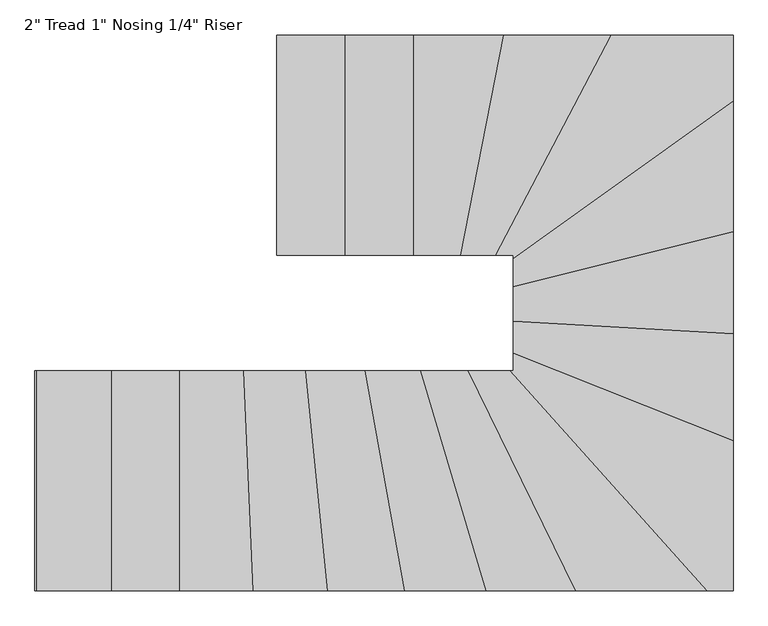
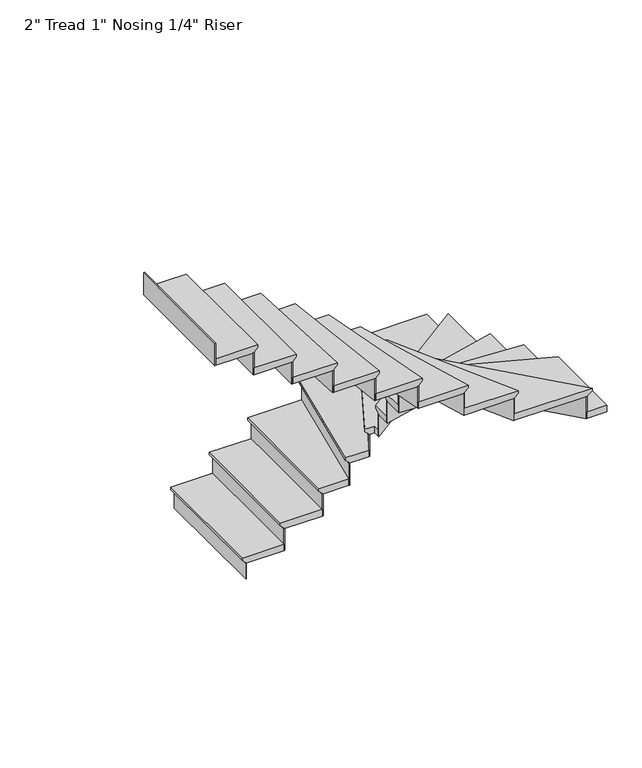
"""IFC4 building model written with IfcOpenShell, lengths in millimetres: stair flight geometry."""

from ifc_helpers import new_model, si_unit, origin, place, context, project, spatial, faceted_brep, source, transform, mapped, element, save


def stair_flight_52755f88(model_context):
    return source(origin(), model_context, "Body", "Brep", [
        faceted_brep([(158.6923968, 2024.0935985, 6551.0833333), (158.6923968, 2024.0935985, 6570.1333333), (158.6923968, 2922.8476133, 6570.1333333), (158.6923968, 2922.8476133, 6551.0833333), (184.0923968, 2024.0935985, 6525.6833333), (184.0923968, 2922.8476133, 6525.6833333), (463.4923968, 2024.0935985, 6570.1333333), (463.4923968, 2922.8476133, 6570.1333333), (184.0923968, 2922.8476133, 6519.3333333), (463.4923968, 2922.8476133, 6519.3333333), (463.4923968, 2024.0935985, 6519.3333333), (184.0923968, 2024.0935985, 6519.3333333)], [[[0, 1, 2, 3]], [[4, 0, 3, 5]], [[2, 1, 6, 7]], [[8, 9, 10, 11]], [[2, 7, 9, 8, 5, 3]], [[8, 11, 4, 5]], [[6, 1, 0, 4, 11, 10]], [[7, 6, 10, 9]]]),
        faceted_brep([(184.0923968, 2024.0935985, 6519.3333333), (184.0923968, 2024.0935985, 6400.8), (190.4423968, 2024.0935985, 6400.8), (190.4423968, 2024.0935985, 6519.3333333), (184.0923968, 2922.8476133, 6519.3333333), (190.4423968, 2922.8476133, 6519.3333333), (190.4423968, 2922.8476133, 6400.8), (184.0923968, 2922.8476133, 6400.8)], [[[0, 1, 2, 3]], [[4, 5, 6, 7]], [[1, 0, 4, 7]], [[2, 1, 7, 6]], [[3, 2, 6, 5]], [[0, 3, 5, 4]]]),
        faceted_brep([(463.4923968, 2024.0935985, 6688.6666667), (463.4923968, 2024.0935985, 6519.3333333), (469.8423968, 2024.0935985, 6519.3333333), (469.8423968, 2024.0935985, 6688.6666667), (463.4923968, 2922.8476133, 6688.6666667), (469.8423968, 2922.8476133, 6688.6666667), (469.8423968, 2922.8476133, 6519.3333333), (463.4923968, 2922.8476133, 6519.3333333)], [[[0, 1, 2, 3]], [[4, 5, 6, 7]], [[1, 0, 4, 7]], [[2, 1, 7, 6]], [[3, 2, 6, 5]], [[0, 3, 5, 4]]]),
        faceted_brep([(438.0923968, 2922.8476133, 6739.4666667), (438.0923968, 2024.0935985, 6739.4666667), (742.8923968, 2024.0935985, 6739.4666667), (742.8923968, 2922.8476133, 6739.4666667), (463.4923968, 2922.8476133, 6688.6666667), (742.8923968, 2922.8476133, 6688.6666667), (742.8923968, 2024.0935985, 6688.6666667), (463.4923968, 2024.0935985, 6688.6666667), (463.4923968, 2922.8476133, 6695.0166667), (438.0923968, 2922.8476133, 6720.4166667), (463.4923968, 2024.0935985, 6695.0166667), (438.0923968, 2024.0935985, 6720.4166667)], [[[0, 1, 2, 3]], [[4, 5, 6, 7]], [[0, 3, 5, 4, 8, 9]], [[4, 7, 10, 8]], [[2, 1, 11, 10, 7, 6]], [[3, 2, 6, 5]], [[11, 1, 0, 9]], [[10, 11, 9, 8]]]),
        faceted_brep([(742.8923968, 2024.0935985, 6858.0), (742.8923968, 2024.0935985, 6688.6666667), (749.2423968, 2024.0935985, 6688.6666667), (749.2423968, 2024.0935985, 6858.0), (742.8923968, 2922.8476133, 6858.0), (749.2423968, 2922.8476133, 6858.0), (749.2423968, 2922.8476133, 6688.6666667), (742.8923968, 2922.8476133, 6688.6666667)], [[[0, 1, 2, 3]], [[4, 5, 6, 7]], [[1, 0, 4, 7]], [[2, 1, 7, 6]], [[3, 2, 6, 5]], [[0, 3, 5, 4]]]),
        faceted_brep([(717.4923968, 2922.8476133, 6908.8), (717.4923968, 2024.0935985, 6908.8), (934.4682952, 2024.0935985, 6908.8), (1111.0881205, 2922.8476133, 6908.8), (742.8923968, 2922.8476133, 6858.0), (1111.0881205, 2922.8476133, 6858.0), (934.4682952, 2024.0935985, 6858.0), (742.8923968, 2024.0935985, 6858.0), (742.8923968, 2922.8476133, 6864.35), (717.4923968, 2922.8476133, 6889.75), (742.8923968, 2024.0935985, 6864.35), (717.4923968, 2024.0935985, 6889.75)], [[[0, 1, 2, 3]], [[4, 5, 6, 7]], [[0, 3, 5, 4, 8, 9]], [[4, 7, 10, 8]], [[2, 1, 11, 10, 7, 6]], [[3, 2, 6, 5]], [[11, 1, 0, 9]], [[10, 11, 9, 8]]]),
        faceted_brep([(934.4682952, 2024.0935985, 7027.3333333), (934.4682952, 2024.0935985, 6858.0), (940.939748, 2024.0935985, 6858.0), (940.939748, 2024.0935985, 7027.3333333), (1111.0881205, 2922.8476133, 7027.3333333), (1117.5595733, 2922.8476133, 7027.3333333), (1117.5595733, 2922.8476133, 6858.0), (1111.0881205, 2922.8476133, 6858.0)], [[[0, 1, 2, 3]], [[4, 5, 6, 7]], [[1, 0, 4, 7]], [[2, 1, 7, 6]], [[3, 2, 6, 5]], [[0, 3, 5, 4]]]),
        faceted_brep([(1085.2023094, 2922.8476133, 7078.1333333), (908.5824841, 2024.0935985, 7078.1333333), (1081.601446, 2024.0935985, 7078.1333333), (1553.5566487, 2922.8476133, 7078.1333333), (1111.0881205, 2922.8476133, 7027.3333333), (1553.5566487, 2922.8476133, 7027.3333333), (1081.601446, 2024.0935985, 7027.3333333), (934.4682952, 2024.0935985, 7027.3333333), (1111.0881205, 2922.8476133, 7033.6833333), (1085.2023094, 2922.8476133, 7059.0833333), (934.4682952, 2024.0935985, 7033.6833333), (908.5824841, 2024.0935985, 7059.0833333)], [[[0, 1, 2, 3]], [[4, 5, 6, 7]], [[0, 3, 5, 4, 8, 9]], [[4, 7, 10, 8]], [[2, 1, 11, 10, 7, 6]], [[3, 2, 6, 5]], [[11, 1, 0, 9]], [[10, 11, 9, 8]]]),
        faceted_brep([(1081.601446, 2024.0935985, 7196.6666667), (1081.601446, 2024.0935985, 7027.3333333), (1088.7737218, 2024.0935985, 7027.3333333), (1088.7737218, 2024.0935985, 7196.6666667), (1553.5566487, 2922.8476133, 7196.6666667), (1560.7289245, 2922.8476133, 7196.6666667), (1560.7289245, 2922.8476133, 7027.3333333), (1553.5566487, 2922.8476133, 7027.3333333)], [[[0, 1, 2, 3]], [[4, 5, 6, 7]], [[1, 0, 4, 7]], [[2, 1, 7, 6]], [[3, 2, 6, 5]], [[0, 3, 5, 4]]]),
        faceted_brep([(2022.1441983, 2621.1058304, 7247.4666667), (2022.1441983, 2922.8476133, 7247.4666667), (1524.8675453, 2922.8476133, 7247.4666667), (1052.9123426, 2024.0935985, 7247.4666667), (1123.3901835, 2024.0935985, 7247.4666667), (1123.3901835, 1978.1363323, 7247.4666667), (2022.1441983, 2922.8476133, 7196.6666667), (2022.1441983, 2621.1058304, 7196.6666667), (1123.3901835, 1978.1363323, 7196.6666667), (1123.3901835, 2024.0935985, 7196.6666667), (1081.601446, 2024.0935985, 7196.6666667), (1553.5566487, 2922.8476133, 7196.6666667), (1081.601446, 2024.0935985, 7203.0166667), (1553.5566487, 2922.8476133, 7203.0166667), (1052.9123426, 2024.0935985, 7228.4166667), (1524.8675453, 2922.8476133, 7228.4166667)], [[[0, 1, 2, 3, 4, 5]], [[6, 7, 8, 9, 10, 11]], [[1, 0, 7, 6]], [[11, 10, 12, 13]], [[4, 3, 14, 12, 10, 9]], [[0, 5, 8, 7]], [[14, 3, 2, 15]], [[12, 14, 15, 13]], [[5, 4, 9, 8]], [[2, 1, 6, 11, 13, 15]]]),
        faceted_brep([(1123.3901835, 1978.1363323, 7366.0), (1123.3901835, 1978.1363323, 7196.6666667), (1123.3901835, 1970.328676, 7196.6666667), (1123.3901835, 1970.328676, 7366.0), (2022.1441983, 2621.1058304, 7366.0), (2022.1441983, 2613.298174, 7366.0), (2022.1441983, 2613.298174, 7196.6666667), (2022.1441983, 2621.1058304, 7196.6666667)], [[[0, 1, 2, 3]], [[4, 5, 6, 7]], [[1, 0, 4, 7]], [[2, 1, 7, 6]], [[3, 2, 6, 5]], [[0, 3, 5, 4]]]),
        faceted_brep([(2022.1441983, 2652.3364556, 7416.8), (1123.3901835, 2009.3669576, 7416.8), (1123.3901835, 1868.1880985, 7416.8), (2022.1441983, 2093.75794, 7416.8), (2022.1441983, 2621.1058304, 7366.0), (2022.1441983, 2093.75794, 7366.0), (1123.3901835, 1868.1880985, 7366.0), (1123.3901835, 1978.1363323, 7366.0), (2022.1441983, 2621.1058304, 7372.35), (2022.1441983, 2652.3364556, 7397.75), (1123.3901835, 1978.1363323, 7372.35), (1123.3901835, 2009.3669576, 7397.75)], [[[0, 1, 2, 3]], [[4, 5, 6, 7]], [[0, 3, 5, 4, 8, 9]], [[4, 7, 10, 8]], [[2, 1, 11, 10, 7, 6]], [[3, 2, 6, 5]], [[11, 1, 0, 9]], [[10, 11, 9, 8]]]),
        faceted_brep([(1123.3901835, 1868.1880985, 7535.3333333), (1123.3901835, 1868.1880985, 7366.0), (1123.3901835, 1861.6411553, 7366.0), (1123.3901835, 1861.6411553, 7535.3333333), (2022.1441983, 2093.75794, 7535.3333333), (2022.1441983, 2087.2109968, 7535.3333333), (2022.1441983, 2087.2109968, 7366.0), (2022.1441983, 2093.75794, 7366.0)], [[[0, 1, 2, 3]], [[4, 5, 6, 7]], [[1, 0, 4, 7]], [[2, 1, 7, 6]], [[3, 2, 6, 5]], [[0, 3, 5, 4]]]),
        faceted_brep([(2022.1441983, 2119.9457129, 7586.1333333), (1123.3901835, 1894.3758714, 7586.1333333), (1123.3901835, 1727.7101185, 7586.1333333), (2022.1441983, 1676.930447, 7586.1333333), (2022.1441983, 2093.75794, 7535.3333333), (2022.1441983, 1676.930447, 7535.3333333), (1123.3901835, 1727.7101185, 7535.3333333), (1123.3901835, 1868.1880985, 7535.3333333), (2022.1441983, 2093.75794, 7541.6833333), (2022.1441983, 2119.9457129, 7567.0833333), (1123.3901835, 1868.1880985, 7541.6833333), (1123.3901835, 1894.3758714, 7567.0833333)], [[[0, 1, 2, 3]], [[4, 5, 6, 7]], [[0, 3, 5, 4, 8, 9]], [[4, 7, 10, 8]], [[2, 1, 11, 10, 7, 6]], [[3, 2, 6, 5]], [[11, 1, 0, 9]], [[10, 11, 9, 8]]]),
        faceted_brep([(1123.3901835, 1727.7101185, 7704.6666667), (1123.3901835, 1727.7101185, 7535.3333333), (1123.3901835, 1721.3499912, 7535.3333333), (1123.3901835, 1721.3499912, 7704.6666667), (2022.1441983, 1676.930447, 7704.6666667), (2022.1441983, 1670.5703197, 7704.6666667), (2022.1441983, 1670.5703197, 7535.3333333), (2022.1441983, 1676.930447, 7535.3333333)], [[[0, 1, 2, 3]], [[4, 5, 6, 7]], [[1, 0, 4, 7]], [[2, 1, 7, 6]], [[3, 2, 6, 5]], [[0, 3, 5, 4]]]),
        faceted_brep([(2022.1441983, 1702.3709564, 7755.4666667), (1123.3901835, 1753.1506279, 7755.4666667), (1123.3901835, 1594.7393557, 7755.4666667), (2022.1441983, 1238.4229709, 7755.4666667), (2022.1441983, 1676.930447, 7704.6666667), (2022.1441983, 1238.4229709, 7704.6666667), (1123.3901835, 1594.7393557, 7704.6666667), (1123.3901835, 1727.7101185, 7704.6666667), (2022.1441983, 1676.930447, 7711.0166667), (2022.1441983, 1702.3709564, 7736.4166667), (1123.3901835, 1727.7101185, 7711.0166667), (1123.3901835, 1753.1506279, 7736.4166667)], [[[0, 1, 2, 3]], [[4, 5, 6, 7]], [[0, 3, 5, 4, 8, 9]], [[4, 7, 10, 8]], [[3, 2, 6, 5]], [[11, 1, 0, 9]], [[10, 11, 9, 8]], [[2, 1, 11, 10, 7, 6]]]),
        faceted_brep([(1123.3901835, 1594.7393557, 7874.0), (1123.3901835, 1594.7393557, 7704.6666667), (1123.3901835, 1587.9085225, 7704.6666667), (1123.3901835, 1587.9085225, 7874.0), (2022.1441983, 1238.4229709, 7874.0), (2022.1441983, 1231.5921376, 7874.0), (2022.1441983, 1231.5921376, 7704.6666667), (2022.1441983, 1238.4229709, 7704.6666667)], [[[0, 1, 2, 3]], [[4, 5, 6, 7]], [[1, 0, 4, 7]], [[2, 1, 7, 6]], [[3, 2, 6, 5]], [[0, 3, 5, 4]]]),
        faceted_brep([(1880.1651285, 652.4935985, 7924.8), (2022.1441983, 652.4935985, 7924.8), (2022.1441983, 1265.7463038, 7924.8), (1123.3901835, 1622.0626887, 7924.8), (1123.3901835, 1551.2476133, 7924.8), (1076.3040211, 1551.2476133, 7924.8), (2022.1441983, 652.4935985, 7874.0), (1880.1651285, 652.4935985, 7874.0), (1076.3040211, 1551.2476133, 7874.0), (1123.3901835, 1551.2476133, 7874.0), (1123.3901835, 1594.7393557, 7874.0), (2022.1441983, 1238.4229709, 7874.0), (1123.3901835, 1594.7393557, 7880.35), (2022.1441983, 1238.4229709, 7880.35), (1123.3901835, 1622.0626887, 7905.75), (2022.1441983, 1265.7463038, 7905.75)], [[[0, 1, 2, 3, 4, 5]], [[6, 7, 8, 9, 10, 11]], [[1, 0, 7, 6]], [[11, 10, 12, 13]], [[4, 3, 14, 12, 10, 9]], [[0, 5, 8, 7]], [[14, 3, 2, 15]], [[12, 14, 15, 13]], [[2, 1, 6, 11, 13, 15]], [[5, 4, 9, 8]]]),
        faceted_brep([(1076.3040211, 1551.2476133, 8043.3333333), (1076.3040211, 1551.2476133, 7874.0), (1067.7846442, 1551.2476133, 7874.0), (1067.7846442, 1551.2476133, 8043.3333333), (1880.1651285, 652.4935985, 8043.3333333), (1871.6457515, 652.4935985, 8043.3333333), (1871.6457515, 652.4935985, 7874.0), (1880.1651285, 652.4935985, 7874.0)], [[[0, 1, 2, 3]], [[4, 5, 6, 7]], [[1, 0, 4, 7]], [[2, 1, 7, 6]], [[3, 2, 6, 5]], [[0, 3, 5, 4]]]),
        faceted_brep([(1914.2426364, 652.4935985, 8094.1333333), (1110.381529, 1551.2476133, 8094.1333333), (909.9761874, 1551.2476133, 8094.1333333), (1349.6820711, 652.4935985, 8094.1333333), (1880.1651285, 652.4935985, 8043.3333333), (1349.6820711, 652.4935985, 8043.3333333), (909.9761874, 1551.2476133, 8043.3333333), (1076.3040211, 1551.2476133, 8043.3333333), (1880.1651285, 652.4935985, 8049.6833333), (1914.2426364, 652.4935985, 8075.0833333), (1076.3040211, 1551.2476133, 8049.6833333), (1110.381529, 1551.2476133, 8075.0833333)], [[[0, 1, 2, 3]], [[4, 5, 6, 7]], [[0, 3, 5, 4, 8, 9]], [[4, 7, 10, 8]], [[2, 1, 11, 10, 7, 6]], [[3, 2, 6, 5]], [[11, 1, 0, 9]], [[10, 11, 9, 8]]]),
        faceted_brep([(909.9761874, 1551.2476133, 8212.6666667), (909.9761874, 1551.2476133, 8043.3333333), (902.9069653, 1551.2476133, 8043.3333333), (902.9069653, 1551.2476133, 8212.6666667), (1349.6820711, 652.4935985, 8212.6666667), (1342.6128491, 652.4935985, 8212.6666667), (1342.6128491, 652.4935985, 8043.3333333), (1349.6820711, 652.4935985, 8043.3333333)], [[[0, 1, 2, 3]], [[4, 5, 6, 7]], [[1, 0, 4, 7]], [[2, 1, 7, 6]], [[3, 2, 6, 5]], [[0, 3, 5, 4]]]),
        faceted_brep([(1377.9589592, 652.4935985, 8263.4666667), (938.2530755, 1551.2476133, 8263.4666667), (717.8211109, 1551.2476133, 8263.4666667), (985.3279709, 652.4935985, 8263.4666667), (1349.6820711, 652.4935985, 8212.6666667), (985.3279709, 652.4935985, 8212.6666667), (717.8211109, 1551.2476133, 8212.6666667), (909.9761874, 1551.2476133, 8212.6666667), (1349.6820711, 652.4935985, 8219.0166667), (1377.9589592, 652.4935985, 8244.4166667), (909.9761874, 1551.2476133, 8219.0166667), (938.2530755, 1551.2476133, 8244.4166667)], [[[0, 1, 2, 3]], [[4, 5, 6, 7]], [[0, 3, 5, 4, 8, 9]], [[4, 7, 10, 8]], [[2, 1, 11, 10, 7, 6]], [[3, 2, 6, 5]], [[11, 1, 0, 9]], [[10, 11, 9, 8]]]),
        faceted_brep([(717.8211109, 1551.2476133, 8382.0), (717.8211109, 1551.2476133, 8212.6666667), (711.1958034, 1551.2476133, 8212.6666667), (711.1958034, 1551.2476133, 8382.0), (985.3279709, 652.4935985, 8382.0), (978.7026634, 652.4935985, 8382.0), (978.7026634, 652.4935985, 8212.6666667), (985.3279709, 652.4935985, 8212.6666667)], [[[0, 1, 2, 3]], [[4, 5, 6, 7]], [[1, 0, 4, 7]], [[2, 1, 7, 6]], [[3, 2, 6, 5]], [[0, 3, 5, 4]]]),
        faceted_brep([(1011.8292006, 652.4935985, 8432.8), (744.3223406, 1551.2476133, 8432.8), (491.9145253, 1551.2476133, 8432.8), (653.8193232, 652.4935985, 8432.8), (985.3279709, 652.4935985, 8382.0), (653.8193232, 652.4935985, 8382.0), (491.9145253, 1551.2476133, 8382.0), (717.8211109, 1551.2476133, 8382.0), (985.3279709, 652.4935985, 8388.35), (1011.8292006, 652.4935985, 8413.75), (717.8211109, 1551.2476133, 8388.35), (744.3223406, 1551.2476133, 8413.75)], [[[0, 1, 2, 3]], [[4, 5, 6, 7]], [[0, 3, 5, 4, 8, 9]], [[4, 7, 10, 8]], [[2, 1, 11, 10, 7, 6]], [[3, 2, 6, 5]], [[11, 1, 0, 9]], [[10, 11, 9, 8]]]),
        faceted_brep([(491.9145253, 1551.2476133, 8551.3333333), (491.9145253, 1551.2476133, 8382.0), (485.4623137, 1551.2476133, 8382.0), (485.4623137, 1551.2476133, 8551.3333333), (653.8193232, 652.4935985, 8551.3333333), (647.3671116, 652.4935985, 8551.3333333), (647.3671116, 652.4935985, 8382.0), (653.8193232, 652.4935985, 8382.0)], [[[0, 1, 2, 3]], [[4, 5, 6, 7]], [[1, 0, 4, 7]], [[2, 1, 7, 6]], [[3, 2, 6, 5]], [[0, 3, 5, 4]]]),
        faceted_brep([(679.6281696, 652.4935985, 8602.1333333), (517.7233717, 1551.2476133, 8602.1333333), (248.510664, 1551.2476133, 8602.1333333), (338.9841344, 652.4935985, 8602.1333333), (653.8193232, 652.4935985, 8551.3333333), (338.9841344, 652.4935985, 8551.3333333), (248.510664, 1551.2476133, 8551.3333333), (491.9145253, 1551.2476133, 8551.3333333), (653.8193232, 652.4935985, 8557.6833333), (679.6281696, 652.4935985, 8583.0833333), (491.9145253, 1551.2476133, 8557.6833333), (517.7233717, 1551.2476133, 8583.0833333)], [[[0, 1, 2, 3]], [[4, 5, 6, 7]], [[0, 3, 5, 4, 8, 9]], [[4, 7, 10, 8]], [[2, 1, 11, 10, 7, 6]], [[3, 2, 6, 5]], [[11, 1, 0, 9]], [[10, 11, 9, 8]]]),
        faceted_brep([(248.510664, 1551.2476133, 8720.6666667), (248.510664, 1551.2476133, 8551.3333333), (242.1285711, 1551.2476133, 8551.3333333), (242.1285711, 1551.2476133, 8720.6666667), (338.9841344, 652.4935985, 8720.6666667), (332.6020415, 652.4935985, 8720.6666667), (332.6020415, 652.4935985, 8551.3333333), (338.9841344, 652.4935985, 8551.3333333)], [[[0, 1, 2, 3]], [[4, 5, 6, 7]], [[1, 0, 4, 7]], [[2, 1, 7, 6]], [[3, 2, 6, 5]], [[0, 3, 5, 4]]]),
        faceted_brep([(364.5125059, 652.4935985, 8771.4666667), (274.0390354, 1551.2476133, 8771.4666667), (-5.0166043, 1551.2476133, 8771.4666667), (33.9204942, 652.4935985, 8771.4666667), (338.9841344, 652.4935985, 8720.6666667), (33.9204942, 652.4935985, 8720.6666667), (-5.0166043, 1551.2476133, 8720.6666667), (248.510664, 1551.2476133, 8720.6666667), (338.9841344, 652.4935985, 8727.0166667), (364.5125059, 652.4935985, 8752.4166667), (248.510664, 1551.2476133, 8727.0166667), (274.0390354, 1551.2476133, 8752.4166667)], [[[0, 1, 2, 3]], [[4, 5, 6, 7]], [[0, 3, 5, 4, 8, 9]], [[4, 7, 10, 8]], [[2, 1, 11, 10, 7, 6]], [[3, 2, 6, 5]], [[11, 1, 0, 9]], [[10, 11, 9, 8]]]),
        faceted_brep([(-5.0166043, 1551.2476133, 8890.0), (-5.0166043, 1551.2476133, 8720.6666667), (-11.3725607, 1551.2476133, 8720.6666667), (-11.3725607, 1551.2476133, 8890.0), (33.9204942, 652.4935985, 8890.0), (27.5645378, 652.4935985, 8890.0), (27.5645378, 652.4935985, 8720.6666667), (33.9204942, 652.4935985, 8720.6666667)], [[[0, 1, 2, 3]], [[4, 5, 6, 7]], [[1, 0, 4, 7]], [[2, 1, 7, 6]], [[3, 2, 6, 5]], [[0, 3, 5, 4]]]),
        faceted_brep([(59.3443199, 652.4935985, 8940.8), (20.4072214, 1551.2476133, 8940.8), (-264.9242294, 1551.2476133, 8940.8), (-264.9242294, 652.4935985, 8940.8), (33.9204942, 652.4935985, 8890.0), (-264.9242294, 652.4935985, 8890.0), (-264.9242294, 1551.2476133, 8890.0), (-5.0166043, 1551.2476133, 8890.0), (33.9204942, 652.4935985, 8896.35), (59.3443199, 652.4935985, 8921.75), (-5.0166043, 1551.2476133, 8896.35), (20.4072214, 1551.2476133, 8921.75)], [[[0, 1, 2, 3]], [[4, 5, 6, 7]], [[0, 3, 5, 4, 8, 9]], [[4, 7, 10, 8]], [[2, 1, 11, 10, 7, 6]], [[3, 2, 6, 5]], [[11, 1, 0, 9]], [[10, 11, 9, 8]]]),
        faceted_brep([(-264.9242294, 1551.2476133, 9059.3333333), (-264.9242294, 1551.2476133, 8890.0), (-271.2742294, 1551.2476133, 8890.0), (-271.2742294, 1551.2476133, 9059.3333333), (-264.9242294, 652.4935985, 9059.3333333), (-271.2742294, 652.4935985, 9059.3333333), (-271.2742294, 652.4935985, 8890.0), (-264.9242294, 652.4935985, 8890.0)], [[[0, 1, 2, 3]], [[4, 5, 6, 7]], [[1, 0, 4, 7]], [[2, 1, 7, 6]], [[3, 2, 6, 5]], [[0, 3, 5, 4]]]),
        faceted_brep([(-239.5242294, 652.4935985, 9110.1333333), (-239.5242294, 1551.2476133, 9110.1333333), (-544.3242294, 1551.2476133, 9110.1333333), (-544.3242294, 652.4935985, 9110.1333333), (-264.9242294, 652.4935985, 9059.3333333), (-544.3242294, 652.4935985, 9059.3333333), (-544.3242294, 1551.2476133, 9059.3333333), (-264.9242294, 1551.2476133, 9059.3333333), (-264.9242294, 652.4935985, 9065.6833333), (-239.5242294, 652.4935985, 9091.0833333), (-264.9242294, 1551.2476133, 9065.6833333), (-239.5242294, 1551.2476133, 9091.0833333)], [[[0, 1, 2, 3]], [[4, 5, 6, 7]], [[0, 3, 5, 4, 8, 9]], [[4, 7, 10, 8]], [[2, 1, 11, 10, 7, 6]], [[3, 2, 6, 5]], [[11, 1, 0, 9]], [[10, 11, 9, 8]]]),
        faceted_brep([(-544.3242294, 1551.2476133, 9228.6666667), (-544.3242294, 1551.2476133, 9059.3333333), (-550.6742294, 1551.2476133, 9059.3333333), (-550.6742294, 1551.2476133, 9228.6666667), (-544.3242294, 652.4935985, 9228.6666667), (-550.6742294, 652.4935985, 9228.6666667), (-550.6742294, 652.4935985, 9059.3333333), (-544.3242294, 652.4935985, 9059.3333333)], [[[0, 1, 2, 3]], [[4, 5, 6, 7]], [[1, 0, 4, 7]], [[2, 1, 7, 6]], [[3, 2, 6, 5]], [[0, 3, 5, 4]]]),
        faceted_brep([(-823.7242294, 1551.2476133, 9398.0), (-823.7242294, 1551.2476133, 9228.6666667), (-830.0742294, 1551.2476133, 9228.6666667), (-830.0742294, 1551.2476133, 9398.0), (-823.7242294, 652.4935985, 9398.0), (-830.0742294, 652.4935985, 9398.0), (-830.0742294, 652.4935985, 9228.6666667), (-823.7242294, 652.4935985, 9228.6666667)], [[[0, 1, 2, 3]], [[4, 5, 6, 7]], [[1, 0, 4, 7]], [[2, 1, 7, 6]], [[3, 2, 6, 5]], [[0, 3, 5, 4]]]),
        faceted_brep([(-518.9242294, 652.4935985, 9279.4666667), (-518.9242294, 1551.2476133, 9279.4666667), (-823.7242294, 1551.2476133, 9279.4666667), (-823.7242294, 652.4935985, 9279.4666667), (-544.3242294, 652.4935985, 9228.6666667), (-823.7242294, 652.4935985, 9228.6666667), (-823.7242294, 1551.2476133, 9228.6666667), (-544.3242294, 1551.2476133, 9228.6666667), (-544.3242294, 652.4935985, 9235.0166667), (-518.9242294, 652.4935985, 9260.4166667), (-544.3242294, 1551.2476133, 9235.0166667), (-518.9242294, 1551.2476133, 9260.4166667)], [[[0, 1, 2, 3]], [[4, 5, 6, 7]], [[0, 3, 5, 4, 8, 9]], [[4, 7, 10, 8]], [[2, 1, 11, 10, 7, 6]], [[3, 2, 6, 5]], [[11, 1, 0, 9]], [[10, 11, 9, 8]]]),
    ])


if __name__ == "__main__":
    model = new_model("IFC4")
    model_context = context("Model", 3, world=origin())
    ifc_project = project(units=[si_unit("LENGTHUNIT", "METRE", prefix="MILLI")], contexts=[model_context])
    site = spatial("IfcSite", under=ifc_project)
    building = spatial("IfcBuilding", under=site)
    placement = place(None, origin())
    stair_flight_shape = stair_flight_52755f88(model_context)
    element("IfcStairFlight", 1, ObjectType="2\" Tread 1\" Nosing 1/4\" Riser", at=placement, inside=building, context=model_context, shape_type="MappedRepresentation", body=[
        mapped(stair_flight_shape, transform((0.0, 0.0, 0.0), x_axis=(1.0, 0.0, 0.0), y_axis=(0.0, 1.0, 0.0), z_axis=(0.0, 0.0, 1.0))),
    ])
    save(model, "model.ifc")
